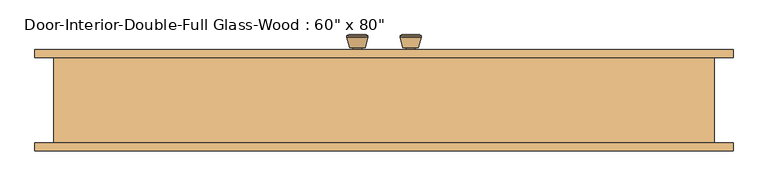
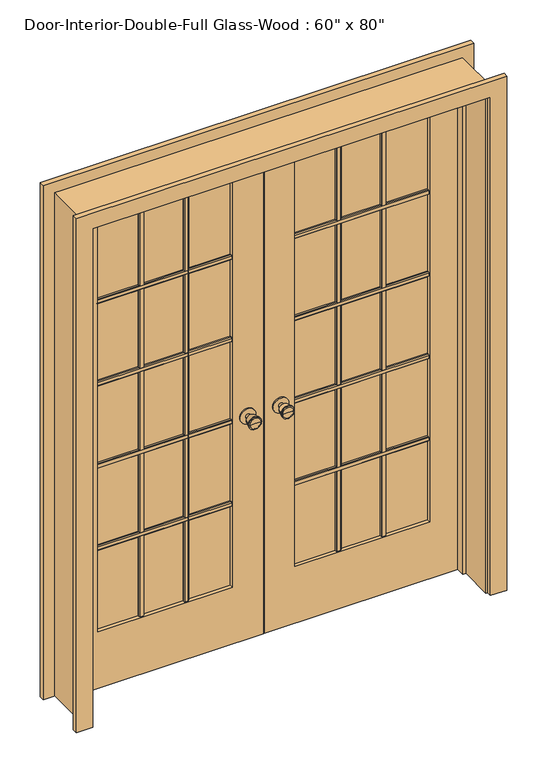
"""IFC4 building model written with IfcOpenShell, lengths in millimetres: door geometry."""

from ifc_helpers import new_model, si_unit, point, frame, frame_2d, origin, place, context, project, spatial, polyline, circle_curve, trimmed, segment, composite_curve, outline, extrude, faceted_brep, source, transform, mapped, element, save
from ifc_brep_helpers import plane_surface, cylinder_surface, revolved_surface, advanced_brep


def door_9d00318c(model_context):
    return source(origin(), model_context, "Body", "SolidModel", [
        advanced_brep(
        [(-63.5, 104.425, 914.4), (-73.5, 104.425, 914.4), (-53.5, 104.425, 914.4), (-83.9758676, 153.425, 914.4), (-63.5, 153.425, 914.4), (-43.0241324, 153.425, 914.4), (-88.5, 151.5971319, 914.4), (-38.5, 151.5971319, 914.4), (-88.5, 148.1334537, 914.4), (-38.5, 148.1334537, 914.4), (-82.136236, 123.425, 914.4), (-44.863764, 123.425, 914.4), (-73.5, 123.425, 914.4), (-53.5, 123.425, 914.4)],
        [
            (0, 1),
            (1, 2, circle_curve(frame((-63.5, 104.425, 914.4), z_axis=(0.0, -1.0, 0.0), x_axis=(1.0, 0.0, 0.0)), 10.0)),
            (2, 0),
            (2, 1, circle_curve(frame((-63.5, 104.425, 914.4), z_axis=(0.0, -1.0, 0.0), x_axis=(1.0, 0.0, 0.0)), 10.0)),
            (3, 4),
            (4, 5),
            (5, 3, circle_curve(frame((-63.5, 153.425, 914.4), z_axis=(0.0, 1.0, 0.0), x_axis=(1.0, 0.0, 0.0)), 20.4758676)),
            (3, 5, circle_curve(frame((-63.5, 153.425, 914.4), z_axis=(0.0, 1.0, 0.0), x_axis=(1.0, 0.0, 0.0)), 20.4758676)),
            (6, 3),
            (5, 7),
            (7, 6, circle_curve(frame((-63.5, 151.5971319, 914.4), z_axis=(0.0, 1.0, 0.0), x_axis=(1.0, 0.0, 0.0)), 25.0)),
            (6, 7, circle_curve(frame((-63.5, 151.5971319, 914.4), z_axis=(0.0, 1.0, 0.0), x_axis=(1.0, 0.0, 0.0)), 25.0)),
            (8, 6),
            (7, 9),
            (9, 8, circle_curve(frame((-63.5, 148.1334537, 914.4), z_axis=(0.0, 1.0, 0.0), x_axis=(1.0, 0.0, 0.0)), 25.0)),
            (8, 9, circle_curve(frame((-63.5, 148.1334537, 914.4), z_axis=(0.0, 1.0, 0.0), x_axis=(1.0, 0.0, 0.0)), 25.0)),
            (10, 8),
            (9, 11),
            (11, 10, circle_curve(frame((-63.5, 123.425, 914.4), z_axis=(0.0, 1.0, 0.0), x_axis=(1.0, 0.0, 0.0)), 18.636236)),
            (10, 11, circle_curve(frame((-63.5, 123.425, 914.4), z_axis=(0.0, 1.0, 0.0), x_axis=(1.0, 0.0, 0.0)), 18.636236)),
            (12, 10),
            (11, 13),
            (13, 12, circle_curve(frame((-63.5, 123.425, 914.4), z_axis=(0.0, 1.0, 0.0), x_axis=(1.0, 0.0, 0.0)), 10.0)),
            (12, 13, circle_curve(frame((-63.5, 123.425, 914.4), z_axis=(0.0, 1.0, 0.0), x_axis=(1.0, 0.0, 0.0)), 10.0)),
            (1, 12),
            (13, 2),
        ],
        [
            plane_surface(frame((-63.5, 104.425, 914.4), z_axis=(0.0, -1.0, 0.0), x_axis=(1.0, 0.0, 0.0))),
            plane_surface(frame((-63.5, 153.425, 914.4), z_axis=(0.0, 1.0, 0.0), x_axis=(1.0, 0.0, 0.0))),
            revolved_surface(polyline([(-43.0241324, 153.425, 914.4), (-38.5, 151.5971319, 914.4)]), (-63.5, 104.425, 914.4), (0.0, -1.0, 0.0)),
            cylinder_surface(frame((-63.5, 104.425, 914.4), z_axis=(0.0, -1.0, 0.0), x_axis=(1.0, 0.0, 0.0)), 25.0),
            revolved_surface(polyline([(-38.5, 148.1334537, 914.4), (-44.863764, 123.425, 914.4)]), (-63.5, 104.425, 914.4), (0.0, -1.0, 0.0)),
            plane_surface(frame((-63.5, 123.425, 914.4), z_axis=(0.0, -1.0, 0.0), x_axis=(1.0, 0.0, 0.0))),
            cylinder_surface(frame((-63.5, 104.425, 914.4), z_axis=(0.0, -1.0, 0.0), x_axis=(1.0, 0.0, 0.0)), 10.0),
        ],
        [
            (0, [[1, 2, 3]]),
            (0, [[-3, 4, -1]]),
            (1, [[5, 6, 7]]),
            (1, [[-6, -5, 8]]),
            (2, [[9, -7, 10, 11]]),
            (2, [[-10, -8, -9, 12]]),
            (3, [[13, -11, 14, 15]]),
            (3, [[-14, -12, -13, 16]]),
            (4, [[17, -15, 18, 19]]),
            (4, [[-18, -16, -17, 20]]),
            (5, [[21, -19, 22, 23]]),
            (5, [[-22, -20, -21, 24]]),
            (6, [[25, -23, 26, -2]]),
            (6, [[-26, -24, -25, -4]]),
        ],
    ),
        extrude(outline(composite_curve([segment(trimmed(circle_curve(frame_2d((914.4, -63.5)), 30.0), [point((914.4, -33.5))], [point((914.4, -93.5))], False, "CARTESIAN"), True, "CONTINUOUS"), segment(trimmed(circle_curve(frame_2d((914.4, -63.5)), 30.0), [point((914.4, -93.5))], [point((914.4, -33.5))], False, "CARTESIAN"), True, "CONTINUOUS")], self_intersect=False)), frame((0.0, 98.425, 0.0), z_axis=(0.0, 1.0, 0.0), x_axis=(0.0, 0.0, 1.0)), (0.0, 0.0, 1.0), 6.0),
        advanced_brep(
        [(-63.5, 57.5, 914.4), (-53.5, 57.5, 914.4), (-73.5, 57.5, 914.4), (-83.9758676, 8.5, 914.4), (-43.0241324, 8.5, 914.4), (-63.5, 8.5, 914.4), (-88.5, 10.3278681, 914.4), (-38.5, 10.3278681, 914.4), (-88.5, 13.7915463, 914.4), (-38.5, 13.7915463, 914.4), (-82.136236, 38.5, 914.4), (-44.863764, 38.5, 914.4), (-73.5, 38.5, 914.4), (-53.5, 38.5, 914.4)],
        [
            (0, 1),
            (1, 2, circle_curve(frame((-63.5, 57.5, 914.4), z_axis=(0.0, 1.0, 0.0), x_axis=(1.0, 0.0, 0.0)), 10.0)),
            (2, 0),
            (2, 1, circle_curve(frame((-63.5, 57.5, 914.4), z_axis=(0.0, 1.0, 0.0), x_axis=(1.0, 0.0, 0.0)), 10.0)),
            (3, 4, circle_curve(frame((-63.5, 8.5, 914.4), z_axis=(0.0, -1.0, 0.0), x_axis=(1.0, 0.0, 0.0)), 20.4758676)),
            (4, 5),
            (5, 3),
            (4, 3, circle_curve(frame((-63.5, 8.5, 914.4), z_axis=(0.0, -1.0, 0.0), x_axis=(1.0, 0.0, 0.0)), 20.4758676)),
            (6, 7, circle_curve(frame((-63.5, 10.3278681, 914.4), z_axis=(0.0, -1.0, 0.0), x_axis=(1.0, 0.0, 0.0)), 25.0)),
            (7, 4),
            (3, 6),
            (7, 6, circle_curve(frame((-63.5, 10.3278681, 914.4), z_axis=(0.0, -1.0, 0.0), x_axis=(1.0, 0.0, 0.0)), 25.0)),
            (8, 9, circle_curve(frame((-63.5, 13.7915463, 914.4), z_axis=(0.0, -1.0, 0.0), x_axis=(1.0, 0.0, 0.0)), 25.0)),
            (9, 7),
            (6, 8),
            (9, 8, circle_curve(frame((-63.5, 13.7915463, 914.4), z_axis=(0.0, -1.0, 0.0), x_axis=(1.0, 0.0, 0.0)), 25.0)),
            (10, 11, circle_curve(frame((-63.5, 38.5, 914.4), z_axis=(0.0, -1.0, 0.0), x_axis=(1.0, 0.0, 0.0)), 18.636236)),
            (11, 9),
            (8, 10),
            (11, 10, circle_curve(frame((-63.5, 38.5, 914.4), z_axis=(0.0, -1.0, 0.0), x_axis=(1.0, 0.0, 0.0)), 18.636236)),
            (12, 13, circle_curve(frame((-63.5, 38.5, 914.4), z_axis=(0.0, -1.0, 0.0), x_axis=(1.0, 0.0, 0.0)), 10.0)),
            (13, 11),
            (10, 12),
            (13, 12, circle_curve(frame((-63.5, 38.5, 914.4), z_axis=(0.0, -1.0, 0.0), x_axis=(1.0, 0.0, 0.0)), 10.0)),
            (1, 13),
            (12, 2),
        ],
        [
            plane_surface(frame((-63.5, 57.5, 914.4), z_axis=(0.0, 1.0, 0.0), x_axis=(1.0, 0.0, 0.0))),
            plane_surface(frame((-63.5, 8.5, 914.4), z_axis=(0.0, -1.0, 0.0), x_axis=(1.0, 0.0, 0.0))),
            revolved_surface(polyline([(-43.0241324, 8.5, 914.4), (-38.5, 10.3278681, 914.4)]), (-63.5, 57.5, 914.4), (0.0, 1.0, 0.0)),
            cylinder_surface(frame((-63.5, 57.5, 914.4), z_axis=(0.0, 1.0, 0.0), x_axis=(1.0, 0.0, 0.0)), 25.0),
            revolved_surface(polyline([(-38.5, 13.7915463, 914.4), (-44.863764, 38.5, 914.4)]), (-63.5, 57.5, 914.4), (0.0, 1.0, 0.0)),
            plane_surface(frame((-63.5, 38.5, 914.4), z_axis=(0.0, 1.0, 0.0), x_axis=(1.0, 0.0, 0.0))),
            cylinder_surface(frame((-63.5, 57.5, 914.4), z_axis=(0.0, 1.0, 0.0), x_axis=(1.0, 0.0, 0.0)), 10.0),
        ],
        [
            (0, [[1, 2, 3]]),
            (0, [[-3, 4, -1]]),
            (1, [[5, 6, 7]]),
            (1, [[8, -7, -6]]),
            (2, [[9, 10, -5, 11]]),
            (2, [[12, -11, -8, -10]]),
            (3, [[13, 14, -9, 15]]),
            (3, [[16, -15, -12, -14]]),
            (4, [[17, 18, -13, 19]]),
            (4, [[20, -19, -16, -18]]),
            (5, [[21, 22, -17, 23]]),
            (5, [[24, -23, -20, -22]]),
            (6, [[-2, 25, -21, 26]]),
            (6, [[-4, -26, -24, -25]]),
        ],
    ),
        extrude(outline(composite_curve([segment(trimmed(circle_curve(frame_2d((914.4, -63.5)), 30.0), [point((914.4, -33.5))], [point((914.4, -93.5))], False, "CARTESIAN"), True, "CONTINUOUS"), segment(trimmed(circle_curve(frame_2d((914.4, -63.5)), 30.0), [point((914.4, -93.5))], [point((914.4, -33.5))], False, "CARTESIAN"), True, "CONTINUOUS")], self_intersect=False)), frame((0.0, 57.5, 0.0), z_axis=(0.0, 1.0, 0.0), x_axis=(0.0, 0.0, 1.0)), (0.0, 0.0, 1.0), 6.0),
        extrude(outline(polyline([(77.47, 1586.23), (77.47, 1567.18), (71.12, 1567.18), (67.945, 1570.355), (67.945, 1583.055), (71.12, 1586.23), (77.47, 1586.23)])), frame((120.65, 0.0, 0.0), z_axis=(1.0, 0.0, 0.0), x_axis=(0.0, 1.0, 0.0)), (0.0, 0.0, 1.0), 520.7),
        extrude(outline(polyline([(77.47, 1249.9975), (77.47, 1230.9475), (71.12, 1230.9475), (67.945, 1234.1225), (67.945, 1246.8225), (71.12, 1249.9975), (77.47, 1249.9975)])), frame((120.65, 0.0, 0.0), z_axis=(1.0, 0.0, 0.0), x_axis=(0.0, 1.0, 0.0)), (0.0, 0.0, 1.0), 520.7),
        extrude(outline(polyline([(77.47, 913.765), (77.47, 894.715), (71.12, 894.715), (67.945, 897.89), (67.945, 910.59), (71.12, 913.765), (77.47, 913.765)])), frame((120.65, 0.0, 0.0), z_axis=(1.0, 0.0, 0.0), x_axis=(0.0, 1.0, 0.0)), (0.0, 0.0, 1.0), 520.7),
        extrude(outline(polyline([(77.47, 577.5325), (77.47, 558.4825), (71.12, 558.4825), (67.945, 561.6575), (67.945, 574.3575), (71.12, 577.5325), (77.47, 577.5325)])), frame((120.65, 0.0, 0.0), z_axis=(1.0, 0.0, 0.0), x_axis=(0.0, 1.0, 0.0)), (0.0, 0.0, 1.0), 520.7),
        extrude(outline(polyline([(458.2583333, 77.47), (477.3083333, 77.47), (477.3083333, 71.12), (474.1333333, 67.945), (461.4333333, 67.945), (458.2583333, 71.12), (458.2583333, 77.47)])), frame((0.0, 0.0, 231.775), z_axis=(0.0, 0.0, 1.0), x_axis=(1.0, 0.0, 0.0)), (0.0, 0.0, 1.0), 1681.1625),
        extrude(outline(polyline([(284.6916667, 77.47), (303.7416667, 77.47), (303.7416667, 71.12), (300.5666667, 67.945), (287.8666667, 67.945), (284.6916667, 71.12), (284.6916667, 77.47)])), frame((0.0, 0.0, 231.775), z_axis=(0.0, 0.0, 1.0), x_axis=(1.0, 0.0, 0.0)), (0.0, 0.0, 1.0), 1681.1625),
        extrude(outline(polyline([(84.455, 1586.23), (90.805, 1586.23), (93.98, 1583.055), (93.98, 1570.355), (90.805, 1567.18), (84.455, 1567.18), (84.455, 1586.23)])), frame((-641.35, 0.0, 0.0), z_axis=(1.0, 0.0, 0.0), x_axis=(0.0, 1.0, 0.0)), (0.0, 0.0, 1.0), 520.7),
        extrude(outline(polyline([(84.455, 1249.9975), (90.805, 1249.9975), (93.98, 1246.8225), (93.98, 1234.1225), (90.805, 1230.9475), (84.455, 1230.9475), (84.455, 1249.9975)])), frame((-641.35, 0.0, 0.0), z_axis=(1.0, 0.0, 0.0), x_axis=(0.0, 1.0, 0.0)), (0.0, 0.0, 1.0), 520.7),
        extrude(outline(polyline([(84.455, 913.765), (90.805, 913.765), (93.98, 910.59), (93.98, 897.89), (90.805, 894.715), (84.455, 894.715), (84.455, 913.765)])), frame((-641.35, 0.0, 0.0), z_axis=(1.0, 0.0, 0.0), x_axis=(0.0, 1.0, 0.0)), (0.0, 0.0, 1.0), 520.7),
        extrude(outline(polyline([(84.455, 577.5325), (90.805, 577.5325), (93.98, 574.3575), (93.98, 561.6575), (90.805, 558.4825), (84.455, 558.4825), (84.455, 577.5325)])), frame((-641.35, 0.0, 0.0), z_axis=(1.0, 0.0, 0.0), x_axis=(0.0, 1.0, 0.0)), (0.0, 0.0, 1.0), 520.7),
        extrude(outline(polyline([(-303.7416667, 84.455), (-303.7416667, 90.805), (-300.5666667, 93.98), (-287.8666667, 93.98), (-284.6916667, 90.805), (-284.6916667, 84.455), (-303.7416667, 84.455)])), frame((0.0, 0.0, 231.775), z_axis=(0.0, 0.0, 1.0), x_axis=(1.0, 0.0, 0.0)), (0.0, 0.0, 1.0), 1681.1625),
        extrude(outline(polyline([(-477.3083333, 84.455), (-477.3083333, 90.805), (-474.1333333, 93.98), (-461.4333333, 93.98), (-458.2583333, 90.805), (-458.2583333, 84.455), (-477.3083333, 84.455)])), frame((0.0, 0.0, 231.775), z_axis=(0.0, 0.0, 1.0), x_axis=(1.0, 0.0, 0.0)), (0.0, 0.0, 1.0), 1681.1625),
        extrude(outline(polyline([(84.455, 1586.23), (90.805, 1586.23), (93.98, 1583.055), (93.98, 1570.355), (90.805, 1567.18), (84.455, 1567.18), (84.455, 1586.23)])), frame((120.65, 0.0, 0.0), z_axis=(1.0, 0.0, 0.0), x_axis=(0.0, 1.0, 0.0)), (0.0, 0.0, 1.0), 520.7),
        extrude(outline(polyline([(84.455, 1249.9975), (90.805, 1249.9975), (93.98, 1246.8225), (93.98, 1234.1225), (90.805, 1230.9475), (84.455, 1230.9475), (84.455, 1249.9975)])), frame((120.65, 0.0, 0.0), z_axis=(1.0, 0.0, 0.0), x_axis=(0.0, 1.0, 0.0)), (0.0, 0.0, 1.0), 520.7),
        extrude(outline(polyline([(84.455, 913.765), (90.805, 913.765), (93.98, 910.59), (93.98, 897.89), (90.805, 894.715), (84.455, 894.715), (84.455, 913.765)])), frame((120.65, 0.0, 0.0), z_axis=(1.0, 0.0, 0.0), x_axis=(0.0, 1.0, 0.0)), (0.0, 0.0, 1.0), 520.7),
        extrude(outline(polyline([(84.455, 577.5325), (90.805, 577.5325), (93.98, 574.3575), (93.98, 561.6575), (90.805, 558.4825), (84.455, 558.4825), (84.455, 577.5325)])), frame((120.65, 0.0, 0.0), z_axis=(1.0, 0.0, 0.0), x_axis=(0.0, 1.0, 0.0)), (0.0, 0.0, 1.0), 520.7),
        extrude(outline(polyline([(458.2583333, 84.455), (458.2583333, 90.805), (461.4333333, 93.98), (474.1333333, 93.98), (477.3083333, 90.805), (477.3083333, 84.455), (458.2583333, 84.455)])), frame((0.0, 0.0, 231.775), z_axis=(0.0, 0.0, 1.0), x_axis=(1.0, 0.0, 0.0)), (0.0, 0.0, 1.0), 1681.1625),
        extrude(outline(polyline([(284.6916667, 84.455), (284.6916667, 90.805), (287.8666667, 93.98), (300.5666667, 93.98), (303.7416667, 90.805), (303.7416667, 84.455), (284.6916667, 84.455)])), frame((0.0, 0.0, 231.775), z_axis=(0.0, 0.0, 1.0), x_axis=(1.0, 0.0, 0.0)), (0.0, 0.0, 1.0), 1681.1625),
        extrude(outline(polyline([(77.47, 1586.23), (77.47, 1567.18), (71.12, 1567.18), (67.945, 1570.355), (67.945, 1583.055), (71.12, 1586.23), (77.47, 1586.23)])), frame((-641.35, 0.0, 0.0), z_axis=(1.0, 0.0, 0.0), x_axis=(0.0, 1.0, 0.0)), (0.0, 0.0, 1.0), 520.7),
        extrude(outline(polyline([(77.47, 1249.9975), (77.47, 1230.9475), (71.12, 1230.9475), (67.945, 1234.1225), (67.945, 1246.8225), (71.12, 1249.9975), (77.47, 1249.9975)])), frame((-641.35, 0.0, 0.0), z_axis=(1.0, 0.0, 0.0), x_axis=(0.0, 1.0, 0.0)), (0.0, 0.0, 1.0), 520.7),
        extrude(outline(polyline([(77.47, 913.765), (77.47, 894.715), (71.12, 894.715), (67.945, 897.89), (67.945, 910.59), (71.12, 913.765), (77.47, 913.765)])), frame((-641.35, 0.0, 0.0), z_axis=(1.0, 0.0, 0.0), x_axis=(0.0, 1.0, 0.0)), (0.0, 0.0, 1.0), 520.7),
        extrude(outline(polyline([(77.47, 577.5325), (77.47, 558.4825), (71.12, 558.4825), (67.945, 561.6575), (67.945, 574.3575), (71.12, 577.5325), (77.47, 577.5325)])), frame((-641.35, 0.0, 0.0), z_axis=(1.0, 0.0, 0.0), x_axis=(0.0, 1.0, 0.0)), (0.0, 0.0, 1.0), 520.7),
        extrude(outline(polyline([(-303.7416667, 77.47), (-284.6916667, 77.47), (-284.6916667, 71.12), (-287.8666667, 67.945), (-300.5666667, 67.945), (-303.7416667, 71.12), (-303.7416667, 77.47)])), frame((0.0, 0.0, 231.775), z_axis=(0.0, 0.0, 1.0), x_axis=(1.0, 0.0, 0.0)), (0.0, 0.0, 1.0), 1681.1625),
        extrude(outline(polyline([(-477.3083333, 77.47), (-458.2583333, 77.47), (-458.2583333, 71.12), (-461.4333333, 67.945), (-474.1333333, 67.945), (-477.3083333, 71.12), (-477.3083333, 77.47)])), frame((0.0, 0.0, 231.775), z_axis=(0.0, 0.0, 1.0), x_axis=(1.0, 0.0, 0.0)), (0.0, 0.0, 1.0), 1681.1625),
        advanced_brep(
        [(63.5, 57.5, 914.4), (73.5, 57.5, 914.4), (53.5, 57.5, 914.4), (83.9758676, 8.5, 914.4), (63.5, 8.5, 914.4), (43.0241324, 8.5, 914.4), (88.5, 10.3278681, 914.4), (38.5, 10.3278681, 914.4), (88.5, 13.7915463, 914.4), (38.5, 13.7915463, 914.4), (82.136236, 38.5, 914.4), (44.863764, 38.5, 914.4), (73.5, 38.5, 914.4), (53.5, 38.5, 914.4)],
        [
            (0, 1),
            (1, 2, circle_curve(frame((63.5, 57.5, 914.4), z_axis=(0.0, 1.0, 0.0), x_axis=(-1.0, 0.0, 0.0)), 10.0)),
            (2, 0),
            (2, 1, circle_curve(frame((63.5, 57.5, 914.4), z_axis=(0.0, 1.0, 0.0), x_axis=(-1.0, 0.0, 0.0)), 10.0)),
            (3, 4),
            (4, 5),
            (5, 3, circle_curve(frame((63.5, 8.5, 914.4), z_axis=(0.0, -1.0, 0.0), x_axis=(-1.0, 0.0, 0.0)), 20.4758676)),
            (3, 5, circle_curve(frame((63.5, 8.5, 914.4), z_axis=(0.0, -1.0, 0.0), x_axis=(-1.0, 0.0, 0.0)), 20.4758676)),
            (6, 3),
            (5, 7),
            (7, 6, circle_curve(frame((63.5, 10.3278681, 914.4), z_axis=(0.0, -1.0, 0.0), x_axis=(-1.0, 0.0, 0.0)), 25.0)),
            (6, 7, circle_curve(frame((63.5, 10.3278681, 914.4), z_axis=(0.0, -1.0, 0.0), x_axis=(-1.0, 0.0, 0.0)), 25.0)),
            (8, 6),
            (7, 9),
            (9, 8, circle_curve(frame((63.5, 13.7915463, 914.4), z_axis=(0.0, -1.0, 0.0), x_axis=(-1.0, 0.0, 0.0)), 25.0)),
            (8, 9, circle_curve(frame((63.5, 13.7915463, 914.4), z_axis=(0.0, -1.0, 0.0), x_axis=(-1.0, 0.0, 0.0)), 25.0)),
            (10, 8),
            (9, 11),
            (11, 10, circle_curve(frame((63.5, 38.5, 914.4), z_axis=(0.0, -1.0, 0.0), x_axis=(-1.0, 0.0, 0.0)), 18.636236)),
            (10, 11, circle_curve(frame((63.5, 38.5, 914.4), z_axis=(0.0, -1.0, 0.0), x_axis=(-1.0, 0.0, 0.0)), 18.636236)),
            (12, 10),
            (11, 13),
            (13, 12, circle_curve(frame((63.5, 38.5, 914.4), z_axis=(0.0, -1.0, 0.0), x_axis=(-1.0, 0.0, 0.0)), 10.0)),
            (12, 13, circle_curve(frame((63.5, 38.5, 914.4), z_axis=(0.0, -1.0, 0.0), x_axis=(-1.0, 0.0, 0.0)), 10.0)),
            (1, 12),
            (13, 2),
        ],
        [
            plane_surface(frame((63.5, 57.5, 914.4), z_axis=(0.0, 1.0, 0.0), x_axis=(-1.0, 0.0, 0.0))),
            plane_surface(frame((63.5, 8.5, 914.4), z_axis=(0.0, -1.0, 0.0), x_axis=(-1.0, 0.0, 0.0))),
            revolved_surface(polyline([(43.0241324, 8.5, 914.4), (38.5, 10.3278681, 914.4)]), (63.5, 57.5, 914.4), (0.0, 1.0, 0.0)),
            cylinder_surface(frame((63.5, 57.5, 914.4), z_axis=(0.0, 1.0, 0.0), x_axis=(-1.0, 0.0, 0.0)), 25.0),
            revolved_surface(polyline([(38.5, 13.7915463, 914.4), (44.863764, 38.5, 914.4)]), (63.5, 57.5, 914.4), (0.0, 1.0, 0.0)),
            plane_surface(frame((63.5, 38.5, 914.4), z_axis=(0.0, 1.0, 0.0), x_axis=(-1.0, 0.0, 0.0))),
            cylinder_surface(frame((63.5, 57.5, 914.4), z_axis=(0.0, 1.0, 0.0), x_axis=(-1.0, 0.0, 0.0)), 10.0),
        ],
        [
            (0, [[1, 2, 3]]),
            (0, [[-3, 4, -1]]),
            (1, [[5, 6, 7]]),
            (1, [[-6, -5, 8]]),
            (2, [[9, -7, 10, 11]]),
            (2, [[-10, -8, -9, 12]]),
            (3, [[13, -11, 14, 15]]),
            (3, [[-14, -12, -13, 16]]),
            (4, [[17, -15, 18, 19]]),
            (4, [[-18, -16, -17, 20]]),
            (5, [[21, -19, 22, 23]]),
            (5, [[-22, -20, -21, 24]]),
            (6, [[25, -23, 26, -2]]),
            (6, [[-26, -24, -25, -4]]),
        ],
    ),
        extrude(outline(composite_curve([segment(trimmed(circle_curve(frame_2d((914.4, 63.5)), 30.0), [point((914.4, 33.5))], [point((914.4, 93.5))], False, "CARTESIAN"), True, "CONTINUOUS"), segment(trimmed(circle_curve(frame_2d((914.4, 63.5)), 30.0), [point((914.4, 93.5))], [point((914.4, 33.5))], False, "CARTESIAN"), True, "CONTINUOUS")], self_intersect=False)), frame((0.0, 57.5, 0.0), z_axis=(0.0, 1.0, 0.0), x_axis=(0.0, 0.0, 1.0)), (0.0, 0.0, 1.0), 6.0),
        advanced_brep(
        [(63.5, 104.425, 914.4), (53.5, 104.425, 914.4), (73.5, 104.425, 914.4), (83.9758676, 153.425, 914.4), (43.0241324, 153.425, 914.4), (63.5, 153.425, 914.4), (88.5, 151.5971319, 914.4), (38.5, 151.5971319, 914.4), (88.5, 148.1334537, 914.4), (38.5, 148.1334537, 914.4), (82.136236, 123.425, 914.4), (44.863764, 123.425, 914.4), (73.5, 123.425, 914.4), (53.5, 123.425, 914.4)],
        [
            (0, 1),
            (1, 2, circle_curve(frame((63.5, 104.425, 914.4), z_axis=(0.0, -1.0, 0.0), x_axis=(-1.0, 0.0, 0.0)), 10.0)),
            (2, 0),
            (2, 1, circle_curve(frame((63.5, 104.425, 914.4), z_axis=(0.0, -1.0, 0.0), x_axis=(-1.0, 0.0, 0.0)), 10.0)),
            (3, 4, circle_curve(frame((63.5, 153.425, 914.4), z_axis=(0.0, 1.0, 0.0), x_axis=(-1.0, 0.0, 0.0)), 20.4758676)),
            (4, 5),
            (5, 3),
            (4, 3, circle_curve(frame((63.5, 153.425, 914.4), z_axis=(0.0, 1.0, 0.0), x_axis=(-1.0, 0.0, 0.0)), 20.4758676)),
            (6, 7, circle_curve(frame((63.5, 151.5971319, 914.4), z_axis=(0.0, 1.0, 0.0), x_axis=(-1.0, 0.0, 0.0)), 25.0)),
            (7, 4),
            (3, 6),
            (7, 6, circle_curve(frame((63.5, 151.5971319, 914.4), z_axis=(0.0, 1.0, 0.0), x_axis=(-1.0, 0.0, 0.0)), 25.0)),
            (8, 9, circle_curve(frame((63.5, 148.1334537, 914.4), z_axis=(0.0, 1.0, 0.0), x_axis=(-1.0, 0.0, 0.0)), 25.0)),
            (9, 7),
            (6, 8),
            (9, 8, circle_curve(frame((63.5, 148.1334537, 914.4), z_axis=(0.0, 1.0, 0.0), x_axis=(-1.0, 0.0, 0.0)), 25.0)),
            (10, 11, circle_curve(frame((63.5, 123.425, 914.4), z_axis=(0.0, 1.0, 0.0), x_axis=(-1.0, 0.0, 0.0)), 18.636236)),
            (11, 9),
            (8, 10),
            (11, 10, circle_curve(frame((63.5, 123.425, 914.4), z_axis=(0.0, 1.0, 0.0), x_axis=(-1.0, 0.0, 0.0)), 18.636236)),
            (12, 13, circle_curve(frame((63.5, 123.425, 914.4), z_axis=(0.0, 1.0, 0.0), x_axis=(-1.0, 0.0, 0.0)), 10.0)),
            (13, 11),
            (10, 12),
            (13, 12, circle_curve(frame((63.5, 123.425, 914.4), z_axis=(0.0, 1.0, 0.0), x_axis=(-1.0, 0.0, 0.0)), 10.0)),
            (1, 13),
            (12, 2),
        ],
        [
            plane_surface(frame((63.5, 104.425, 914.4), z_axis=(0.0, -1.0, 0.0), x_axis=(-1.0, 0.0, 0.0))),
            plane_surface(frame((63.5, 153.425, 914.4), z_axis=(0.0, 1.0, 0.0), x_axis=(-1.0, 0.0, 0.0))),
            revolved_surface(polyline([(43.0241324, 153.425, 914.4), (38.5, 151.5971319, 914.4)]), (63.5, 104.425, 914.4), (0.0, -1.0, 0.0)),
            cylinder_surface(frame((63.5, 104.425, 914.4), z_axis=(0.0, -1.0, 0.0), x_axis=(-1.0, 0.0, 0.0)), 25.0),
            revolved_surface(polyline([(38.5, 148.1334537, 914.4), (44.863764, 123.425, 914.4)]), (63.5, 104.425, 914.4), (0.0, -1.0, 0.0)),
            plane_surface(frame((63.5, 123.425, 914.4), z_axis=(0.0, -1.0, 0.0), x_axis=(-1.0, 0.0, 0.0))),
            cylinder_surface(frame((63.5, 104.425, 914.4), z_axis=(0.0, -1.0, 0.0), x_axis=(-1.0, 0.0, 0.0)), 10.0),
        ],
        [
            (0, [[1, 2, 3]]),
            (0, [[-3, 4, -1]]),
            (1, [[5, 6, 7]]),
            (1, [[8, -7, -6]]),
            (2, [[9, 10, -5, 11]]),
            (2, [[12, -11, -8, -10]]),
            (3, [[13, 14, -9, 15]]),
            (3, [[16, -15, -12, -14]]),
            (4, [[17, 18, -13, 19]]),
            (4, [[20, -19, -16, -18]]),
            (5, [[21, 22, -17, 23]]),
            (5, [[24, -23, -20, -22]]),
            (6, [[-2, 25, -21, 26]]),
            (6, [[-4, -26, -24, -25]]),
        ],
    ),
        extrude(outline(composite_curve([segment(trimmed(circle_curve(frame_2d((914.4, 63.5)), 30.0), [point((914.4, 33.5))], [point((914.4, 93.5))], False, "CARTESIAN"), True, "CONTINUOUS"), segment(trimmed(circle_curve(frame_2d((914.4, 63.5)), 30.0), [point((914.4, 93.5))], [point((914.4, 33.5))], False, "CARTESIAN"), True, "CONTINUOUS")], self_intersect=False)), frame((0.0, 98.425, 0.0), z_axis=(0.0, 1.0, 0.0), x_axis=(0.0, 0.0, 1.0)), (0.0, 0.0, 1.0), 6.0),
        extrude(outline(polyline([(0.0, 768.35), (0.0, 831.85), (2101.85, 831.85), (2101.85, -831.85), (0.0, -831.85), (0.0, -768.35), (2038.35, -768.35), (2038.35, 768.35), (0.0, 768.35)])), frame((0.0, 98.425, 0.0), z_axis=(0.0, 1.0, 0.0), x_axis=(0.0, 0.0, 1.0)), (0.0, 0.0, 1.0), 19.05),
        extrude(outline(polyline([(0.0, 768.35), (0.0, 831.85), (2101.85, 831.85), (2101.85, -831.85), (0.0, -831.85), (0.0, -768.35), (2038.35, -768.35), (2038.35, 768.35), (0.0, 768.35)])), frame((0.0, -123.825, 0.0), z_axis=(0.0, 1.0, 0.0), x_axis=(0.0, 0.0, 1.0)), (0.0, 0.0, 1.0), 19.05),
        extrude(outline(polyline([(2032.0, -762.0), (0.0, -762.0), (0.0, -1.6019111), (2032.0, -1.6019111), (2032.0, -762.0)]), holes=[polyline([(231.775, -641.35), (1912.9375, -641.35), (1912.9375, -120.65), (231.775, -120.65), (231.775, -641.35)])]), frame((0.0, 63.5, 0.0), z_axis=(0.0, 1.0, 0.0), x_axis=(0.0, 0.0, 1.0)), (0.0, 0.0, 1.0), 34.925),
        extrude(outline(polyline([(0.0, 762.0), (2032.0, 762.0), (2032.0, 1.5875), (0.0, 1.5875), (0.0, 762.0)]), holes=[polyline([(1912.9375, 120.65), (1912.9375, 641.35), (231.775, 641.35), (231.775, 120.65), (1912.9375, 120.65)])]), frame((0.0, 63.5, 0.0), z_axis=(0.0, 1.0, 0.0), x_axis=(0.0, 0.0, 1.0)), (0.0, 0.0, 1.0), 34.925),
        faceted_brep([(787.4, 98.425, 0.0), (787.4, -104.775, 0.0), (762.0, -104.775, 0.0), (762.0, 28.575, 0.0), (749.3, 28.575, 0.0), (749.3, 63.5, 0.0), (762.0, 63.5, 0.0), (762.0, 98.425, 0.0), (787.4, 98.425, 2057.4), (787.4, -104.775, 2057.4), (-787.4, -104.775, 2057.4), (-787.4, -104.775, 0.0), (-762.0, -104.775, 0.0), (-762.0, -104.775, 2032.0), (762.0, -104.775, 2032.0), (762.0, 28.575, 2032.0), (-762.0, 28.575, 2032.0), (-762.0, 28.575, 0.0), (-749.3, 28.575, 0.0), (-749.3, 28.575, 2019.3), (749.3, 28.575, 2019.3), (749.3, 63.5, 2019.3), (1.5875, 63.5, 2019.3), (-1.6019111, 63.5, 2019.3), (-749.3, 63.5, 2019.3), (-749.3, 63.5, 0.0), (-762.0, 63.5, 0.0), (-762.0, 63.5, 2032.0), (-1.6019111, 63.5, 2032.0), (1.5875, 63.5, 2032.0), (762.0, 63.5, 2032.0), (762.0, 98.425, 2032.0), (1.5875, 98.425, 2032.0), (-1.6019111, 98.425, 2032.0), (-762.0, 98.425, 2032.0), (-762.0, 98.425, 0.0), (-787.4, 98.425, 0.0), (-787.4, 98.425, 2057.4)], [[[0, 1, 2, 3, 4, 5, 6, 7]], [[1, 0, 8, 9]], [[2, 1, 9, 10, 11, 12, 13, 14]], [[3, 2, 14, 15]], [[4, 3, 15, 16, 17, 18, 19, 20]], [[5, 4, 20, 21]], [[6, 5, 21, 22, 23, 24, 25, 26, 27, 28, 29, 30]], [[7, 6, 30, 31]], [[0, 7, 31, 32, 33, 34, 35, 36, 37, 8]], [[9, 8, 37, 10]], [[14, 13, 16, 15]], [[20, 19, 24, 23, 22, 21]], [[31, 30, 29, 28, 27, 34, 33, 32]], [[12, 11, 36, 35, 26, 25, 18, 17]], [[11, 10, 37, 36]], [[13, 12, 17, 16]], [[19, 18, 25, 24]], [[27, 26, 35, 34]]]),
        extrude(outline(polyline([(641.35, 77.47), (120.65, 77.47), (120.65, 84.455), (641.35, 84.455), (641.35, 77.47)])), frame((0.0, 0.0, 231.775), z_axis=(0.0, 0.0, 1.0), x_axis=(1.0, 0.0, 0.0)), (0.0, 0.0, 1.0), 1681.1625),
        extrude(outline(polyline([(-120.65, 77.47), (-641.35, 77.47), (-641.35, 84.455), (-120.65, 84.455), (-120.65, 77.47)])), frame((0.0, 0.0, 231.775), z_axis=(0.0, 0.0, 1.0), x_axis=(1.0, 0.0, 0.0)), (0.0, 0.0, 1.0), 1681.1625),
    ])


if __name__ == "__main__":
    model = new_model("IFC4")
    model_context = context("Model", 3, world=origin())
    ifc_project = project(units=[si_unit("LENGTHUNIT", "METRE", prefix="MILLI")], contexts=[model_context])
    site = spatial("IfcSite", under=ifc_project)
    building = spatial("IfcBuilding", under=site)
    placement = place(None, origin())
    door_shape = door_9d00318c(model_context)
    element("IfcDoor", 1, ObjectType="Door-Interior-Double-Full Glass-Wood : 60\" x 80\"", at=placement, inside=building, context=model_context, shape_type="MappedRepresentation", body=[
        mapped(door_shape, transform((0.0, 0.0, 0.0), x_axis=(1.0, 0.0, 0.0), y_axis=(0.0, 1.0, 0.0), z_axis=(0.0, 0.0, 1.0))),
    ])
    save(model, "model.ifc")

# Revit data of these elements
# Type "Door-Interior-Double-Full Glass-Wood : 60\" x 80\""
#   Type Mark = "8"
#   Assembly Code = "C1020300"
#   Analytic Construction = "French door, wood frame with single glass"
#   Top Rail = 0' - 4 11/16"
#   Thickness = 0' - 1 3/8"
#   Thermal Resistance (R) = 1.0696 (h·ft²·°F)/BTU
#   Swing Angle [instance default] = 90.00°
#   Stiles = 0' - 4 3/4"
#   Rough Width = 5' - 2"
#   Rough Height = 6' - 9"
#   Panel Width = 2' - 6"
#   Height = 6' - 8"
#   Width = 5' - 0"
#   Heat Transfer Coefficient (U) = 0.9350 BTU/(h·ft²·°F)
#   Bottom Rail = 0' - 9 1/8"
#   Show Grill [instance default] = yes
#   Trim Material = Cherry
#   Panel Material = Cherry
#   Frame Material = Cherry
#   Door Handle Material = Aluminum
#   Visual Light Transmittance = 0
#   Solar Heat Gain Coefficient = 0
#   Wall Closure = (empty or 0)
#   Function = (empty or 0)
# Element 1 (IfcDoor, "Door-Interior-Double-Full Glass-Wood : 60\" x 80\"")
#   Materials on its faces: "Cherry", "Aluminum", "Glass"
# Materials
#   "Cherry": class "Wood", colour RGB 226 177 128, transparency 0, Description = "Prunus Serotina", Cost = 0
#   "Aluminum": class "Metal", colour RGB 247 247 247, transparency 0, Description = "Aluminum 6061", Cost = 0
#   "Glass": class "Glass", colour RGB 0 128 192, transparency 0.75, Description = "Soda Lime Glass", Cost = 0
